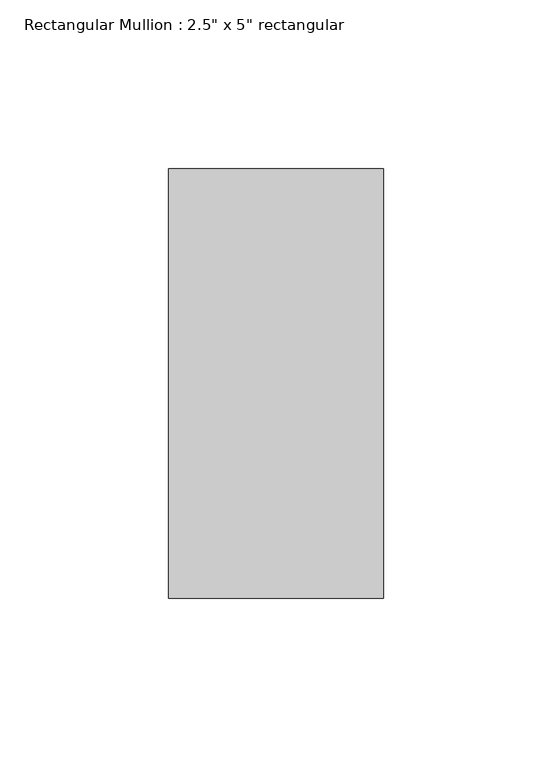
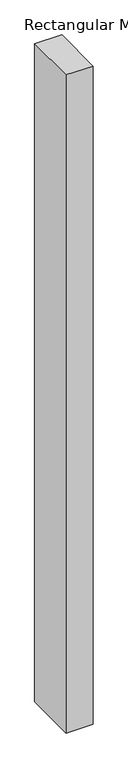
"""IFC4 building model written with IfcOpenShell, lengths in millimetres: member geometry."""

from ifc_helpers import new_model, si_unit, frame, origin, place, context, project, spatial, polyline, outline, extrude, source, transform, mapped, element, save


def member_e04b046a(model_context):
    return source(origin(), model_context, "Body", "SweptSolid", [
        extrude(outline(polyline([(31.75, 63.5), (31.75, -63.5), (-31.75, -63.5), (-31.75, 63.5), (31.75, 63.5)])), frame((0.0, 0.0, -1629.9147167), z_axis=(0.0, 0.0, 1.0), x_axis=(1.0, 0.0, 0.0)), (0.0, 0.0, 1.0), 1629.9147167),
    ])


if __name__ == "__main__":
    model = new_model("IFC4")
    model_context = context("Model", 3, world=origin())
    ifc_project = project(units=[si_unit("LENGTHUNIT", "METRE", prefix="MILLI")], contexts=[model_context])
    site = spatial("IfcSite", under=ifc_project)
    building = spatial("IfcBuilding", under=site)
    placement = place(None, origin())
    member_shape = member_e04b046a(model_context)
    element("IfcMember", 1, ObjectType="Rectangular Mullion : 2.5\" x 5\" rectangular", at=placement, inside=building, context=model_context, shape_type="MappedRepresentation", body=[
        mapped(member_shape, transform((0.0, 0.0, 0.0), x_axis=(1.0, 0.0, 0.0), y_axis=(0.0, 1.0, 0.0), z_axis=(0.0, 0.0, 1.0))),
    ])
    save(model, "model.ifc")

# Revit data of these elements
# Type "Rectangular Mullion : 2.5\" x 5\" rectangular"
#   built-in parameter 1007304 = 0.416667 (stored number, unit not read)
#   built-in parameter 1007301 = 0.104167 (stored number, unit not read)
#   built-in parameter 1007300 = 0.104167 (stored number, unit not read)
# Element 1 (IfcMember, "Rectangular Mullion : 2.5\" x 5\" rectangular")
#   Materials on its faces: "Aluminum"
# Materials
#   "Aluminum": class "Metal", colour RGB 247 247 247, transparency 0, Description = "Aluminum 6061", Cost = 0
